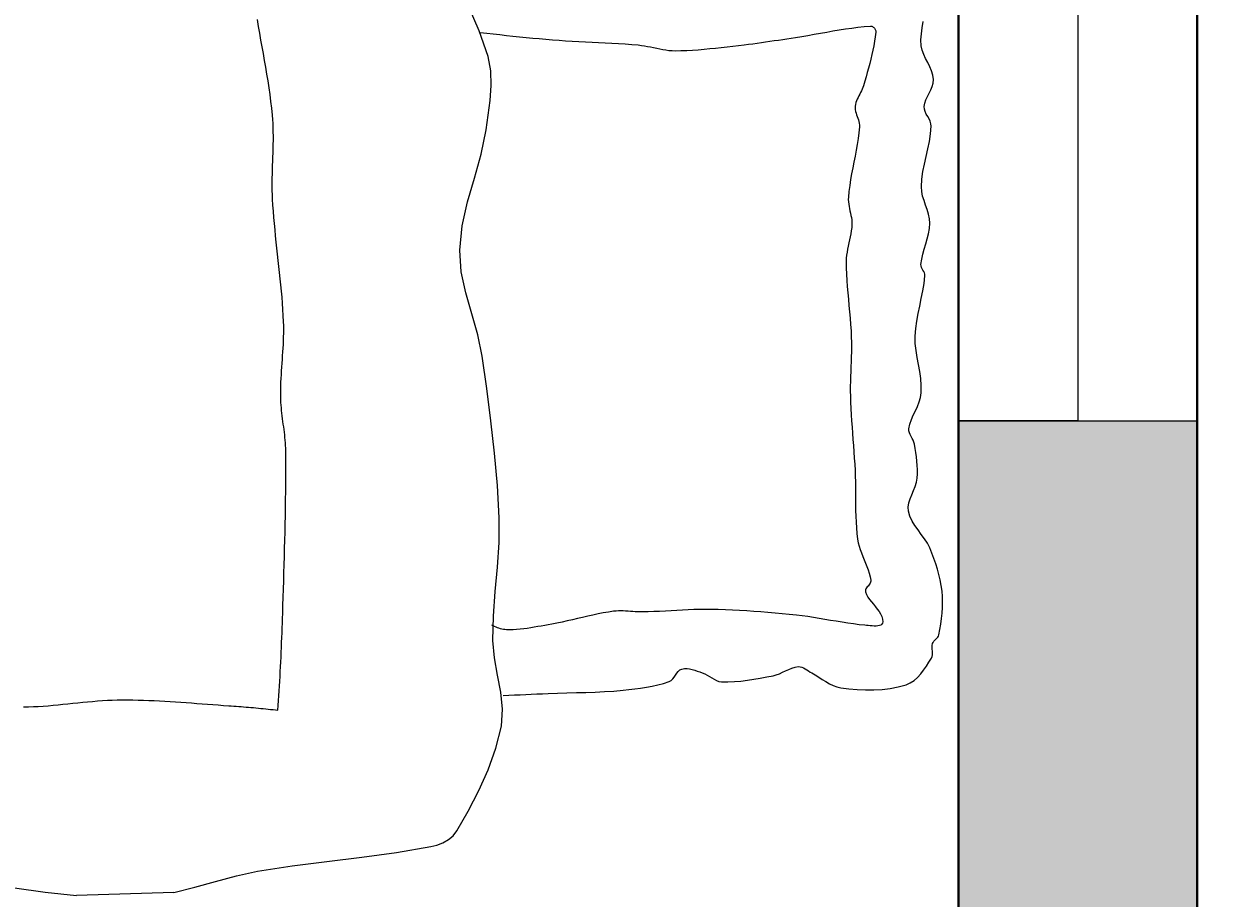
# Model space of a CAD drawing. Units: inches. Extents: x 1441 to 2460, y 1648 to 2683.
# Tile 16 of 35: x 1845 to 1890, y 2058 to 2091. Entities that reach past the tile are written whole.
import ezdxf

# ---------------------------------------------------------------- set-up
doc = ezdxf.new("R2010")
doc.units = ezdxf.units.IN
for name, color, linetype, lineweight in [('A-ANNO-DIMS', 2, 'Continuous', 18), ('A-FURN', 8, 'Continuous', 15), ('A-GLAZ', 4, 'Continuous', 18), ('A-WALL', 7, 'Continuous', 40)]:
    doc.layers.add(name, color=color, linetype=linetype, lineweight=lineweight)
doc.layers.add('A-WALL-PATT', color=251, linetype='Continuous', lineweight=13, true_color=0x636466)
doc.styles.get("Standard").update_dxf_attribs({"font": 'arial.ttf'})
doc.dimstyles.get("Standard").update_dxf_attribs({"dimtxt": 0.18, "dimasz": 0.18, "dimexe": 0.18, "dimexo": 0.0625, "dimgap": 0.09, "dimtad": 0, "dimtih": 1, "dimtoh": 1, "dimdec": 4, "dimzin": 0, "dimdsep": 46, "dimtxsty": 'Standard', "dimcen": 0.09, "dimadec": 0, "dimazin": 0, "dimtfac": 1, "dimtdec": 4, "dimtofl": 0, "dimtmove": 0, "dimatfit": 3, "dimfxl": 1, "dimtolj": 1, "dimtzin": 0, "dimarcsym": 0})

# ---------------------------------------------------------------- blocks, each defined once
blk = doc.blocks.new('BED-DOUBLE-PLAN')
for p, q in [((33.569, 91.32), (33.41, 91.271)), ((33.735, 91.343), (33.569, 91.32)), ((33.867, 91.333), (33.735, 91.343)), ((33.995, 91.298), (33.867, 91.333)), ((34.121, 91.245), (33.995, 91.298)), ((51.797, 91.361), (51.599, 91.285)), ((51.997, 91.432), (51.797, 91.361)), ((52.2, 91.497), (51.997, 91.432)), ((52.404, 91.554), (52.2, 91.497)), ((52.61, 91.603), (52.404, 91.554)), ((52.818, 91.642), (52.61, 91.603)), ((53.027, 91.67), (52.818, 91.642)), ((53.234, 91.686), (53.027, 91.67)), ((53.441, 91.69), (53.234, 91.686)), ((53.649, 91.684), (53.441, 91.69)), ((53.857, 91.67), (53.649, 91.684)), ((54.065, 91.648), (53.857, 91.67)), ((54.272, 91.619), (54.065, 91.648)), ((54.478, 91.587), (54.272, 91.619)), ((54.683, 91.551), (54.478, 91.587)), ((54.729, 91.535), (54.683, 91.551)), ((54.771, 91.509), (54.729, 91.535)), ((54.81, 91.475), (54.771, 91.509)), ((54.847, 91.437), (54.81, 91.475)), ((54.884, 91.398), (54.847, 91.437)), ((54.922, 91.361), (54.884, 91.398)), ((54.963, 91.331), (54.922, 91.361)), ((55.008, 91.31), (54.963, 91.331)), ((55.076, 91.296), (55.008, 91.31)), ((55.147, 91.294), (55.076, 91.296)), ((55.219, 91.299), (55.147, 91.294)), ((55.292, 91.306), (55.219, 91.299)), ((55.364, 91.311), (55.292, 91.306)), ((55.433, 91.31), (55.364, 91.311)), ((55.499, 91.298), (55.433, 91.31)), ((55.56, 91.27), (55.499, 91.298)), ((31.78, 90.922), (31.549, 90.959)), ((32.011, 90.889), (31.78, 90.922)), ((32.24, 90.873), (32.011, 90.889)), ((32.466, 90.885), (32.24, 90.873)), ((32.63, 90.922), (32.466, 90.885)), ((32.789, 90.98), (32.63, 90.922)), ((32.945, 91.051), (32.789, 90.98)), ((33.099, 91.129), (32.945, 91.051)), ((33.253, 91.205), (33.099, 91.129)), ((33.41, 91.271), (33.253, 91.205)), ((34.245, 91.181), (34.121, 91.245)), ((34.37, 91.117), (34.245, 91.181)), ((34.495, 91.058), (34.37, 91.117)), ((34.624, 91.015), (34.495, 91.058)), ((34.756, 90.994), (34.624, 91.015)), ((34.852, 91.003), (34.756, 90.994)), ((34.945, 91.032), (34.852, 91.003)), ((35.036, 91.076), (34.945, 91.032)), ((35.126, 91.127), (35.036, 91.076)), ((35.216, 91.178), (35.126, 91.127)), ((35.307, 91.222), (35.216, 91.178)), ((35.4, 91.252), (35.307, 91.222)), ((35.496, 91.261), (35.4, 91.252)), ((35.784, 91.238), (35.496, 91.261)), ((36.07, 91.194), (35.784, 91.238)), ((36.354, 91.135), (36.07, 91.194)), ((36.638, 91.07), (36.354, 91.135)), ((36.922, 91.006), (36.638, 91.07)), ((37.206, 90.949), (36.922, 91.006)), ((37.492, 90.908), (37.206, 90.949)), ((37.78, 90.89), (37.492, 90.908)), ((37.955, 90.902), (37.78, 90.89)), ((38.128, 90.938), (37.955, 90.902)), ((38.299, 90.989), (38.128, 90.938)), ((38.469, 91.048), (38.299, 90.989)), ((38.639, 91.107), (38.469, 91.048)), ((38.81, 91.159), (38.639, 91.107)), ((38.983, 91.195), (38.81, 91.159)), ((39.158, 91.208), (38.983, 91.195)), ((39.356, 91.195), (39.158, 91.208)), ((39.551, 91.161), (39.356, 91.195)), ((39.744, 91.114), (39.551, 91.161)), ((39.936, 91.058), (39.744, 91.114)), ((40.129, 91), (39.936, 91.058)), ((40.322, 90.946), (40.129, 91)), ((40.516, 90.901), (40.322, 90.946)), ((40.713, 90.873), (40.516, 90.901)), ((40.767, 90.876), (40.713, 90.873)), ((40.821, 90.893), (40.767, 90.876)), ((40.873, 90.918), (40.821, 90.893)), ((40.924, 90.949), (40.873, 90.918)), ((40.975, 90.979), (40.924, 90.949)), ((41.027, 91.005), (40.975, 90.979)), ((41.081, 91.022), (41.027, 91.005)), ((41.135, 91.025), (41.081, 91.022)), ((41.423, 90.993), (41.135, 91.025)), ((41.708, 90.945), (41.423, 90.993)), ((41.993, 90.887), (41.708, 90.945)), ((42.277, 90.826), (41.993, 90.887)), ((45.014, 90.865), (44.748, 90.826)), ((45.28, 90.887), (45.014, 90.865)), ((45.546, 90.884), (45.28, 90.887)), ((45.723, 90.857), (45.546, 90.884)), ((45.894, 90.807), (45.723, 90.857)), ((50.888, 90.886), (50.723, 90.763)), ((51.053, 91.006), (50.888, 90.886)), ((51.224, 91.115), (51.053, 91.006)), ((51.403, 91.204), (51.224, 91.115)), ((51.599, 91.285), (51.403, 91.204)), ((55.709, 91.176), (55.56, 91.27)), ((55.86, 91.078), (55.709, 91.176)), ((56.01, 90.975), (55.86, 91.078)), ((56.153, 90.865), (56.01, 90.975)), ((56.284, 90.746), (56.153, 90.865)), ((42.561, 90.766), (42.277, 90.826)), ((42.845, 90.714), (42.561, 90.766)), ((43.131, 90.675), (42.845, 90.714)), ((43.419, 90.654), (43.131, 90.675)), ((43.686, 90.66), (43.419, 90.654)), ((43.952, 90.687), (43.686, 90.66)), ((44.218, 90.73), (43.952, 90.687)), ((44.483, 90.779), (44.218, 90.73)), ((44.748, 90.826), (44.483, 90.779)), ((46.062, 90.739), (45.894, 90.807)), ((46.228, 90.663), (46.062, 90.739)), ((46.394, 90.585), (46.228, 90.663)), ((46.562, 90.514), (46.394, 90.585)), ((46.733, 90.456), (46.562, 90.514)), ((46.908, 90.42), (46.733, 90.456)), ((46.984, 90.419), (46.908, 90.42)), ((47.057, 90.436), (46.984, 90.419)), ((47.128, 90.465), (47.057, 90.436)), ((47.199, 90.502), (47.128, 90.465)), ((47.27, 90.541), (47.199, 90.502)), ((47.342, 90.578), (47.27, 90.541)), ((47.415, 90.609), (47.342, 90.578)), ((47.49, 90.629), (47.415, 90.609)), ((47.648, 90.655), (47.49, 90.629)), ((47.807, 90.68), (47.648, 90.655)), ((47.967, 90.702), (47.807, 90.68)), ((48.127, 90.721), (47.967, 90.702)), ((48.287, 90.734), (48.127, 90.721)), ((48.447, 90.741), (48.287, 90.734)), ((48.607, 90.741), (48.447, 90.741)), ((48.767, 90.731), (48.607, 90.741)), ((48.926, 90.703), (48.767, 90.731)), ((49.084, 90.654), (48.926, 90.703)), ((49.24, 90.592), (49.084, 90.654)), ((49.395, 90.526), (49.24, 90.592)), ((49.549, 90.466), (49.395, 90.526)), ((49.704, 90.42), (49.549, 90.466)), ((49.861, 90.397), (49.704, 90.42)), ((50.019, 90.406), (49.861, 90.397)), ((50.209, 90.459), (50.019, 90.406)), ((50.387, 90.542), (50.209, 90.459)), ((50.558, 90.646), (50.387, 90.542)), ((50.723, 90.763), (50.558, 90.646)), ((56.399, 90.616), (56.284, 90.746)), ((56.493, 90.473), (56.399, 90.616)), ((56.561, 90.317), (56.493, 90.473)), ((56.643, 90.02), (56.561, 90.317)), ((56.701, 89.716), (56.643, 90.02)), ((56.736, 89.408), (56.701, 89.716)), ((31.729, 89.025), (31.74, 89.05)), ((31.74, 89.05), (31.755, 89.074)), ((31.755, 89.074), (31.774, 89.097)), ((31.774, 89.097), (31.795, 89.117)), ((31.795, 89.117), (31.818, 89.136)), ((31.818, 89.136), (31.843, 89.151)), ((31.843, 89.151), (31.869, 89.163)), ((31.869, 89.163), (31.896, 89.172)), ((31.896, 89.172), (31.922, 89.176)), ((31.922, 89.176), (31.948, 89.176)), ((31.948, 89.176), (32.119, 89.153)), ((32.119, 89.153), (32.29, 89.126)), ((32.29, 89.126), (32.459, 89.095)), ((32.459, 89.095), (32.629, 89.06)), ((32.629, 89.06), (32.797, 89.023)), ((53.438, 89.006), (53.527, 89.081)), ((53.527, 89.081), (53.616, 89.156)), ((53.616, 89.156), (53.705, 89.228)), ((53.705, 89.228), (53.796, 89.294)), ((53.796, 89.294), (53.889, 89.351)), ((53.889, 89.351), (53.985, 89.396)), ((53.985, 89.396), (54.086, 89.424)), ((54.086, 89.424), (54.192, 89.433)), ((54.192, 89.433), (54.243, 89.423)), ((54.243, 89.423), (54.282, 89.397)), ((54.282, 89.397), (54.31, 89.358)), ((54.31, 89.358), (54.329, 89.307)), ((54.329, 89.307), (54.341, 89.247)), ((54.341, 89.247), (54.346, 89.18)), ((54.346, 89.109), (54.342, 89.035)), ((54.346, 89.18), (54.346, 89.109)), ((56.752, 89.096), (56.736, 89.408)), ((56.751, 88.783), (56.752, 89.096)), ((31.722, 88.975), (31.723, 89)), ((31.741, 88.737), (31.722, 88.975)), ((31.723, 89), (31.729, 89.025)), ((31.765, 88.499), (31.741, 88.737)), ((32.797, 89.023), (32.966, 88.982)), ((32.966, 88.982), (33.133, 88.94)), ((33.133, 88.94), (33.301, 88.895)), ((33.301, 88.895), (33.468, 88.85)), ((33.468, 88.85), (33.635, 88.803)), ((33.635, 88.803), (33.801, 88.756)), ((33.801, 88.756), (33.968, 88.709)), ((33.968, 88.709), (34.034, 88.688)), ((34.034, 88.688), (34.099, 88.662)), ((34.099, 88.662), (34.162, 88.632)), ((34.162, 88.632), (34.225, 88.599)), ((34.225, 88.599), (34.288, 88.566)), ((51.463, 88.586), (51.591, 88.632)), ((51.591, 88.632), (51.719, 88.683)), ((51.719, 88.683), (51.846, 88.735)), ((51.846, 88.735), (51.972, 88.787)), ((51.972, 88.787), (52.1, 88.838)), ((52.1, 88.838), (52.228, 88.885)), ((52.228, 88.885), (52.357, 88.926)), ((52.357, 88.926), (52.488, 88.961)), ((52.488, 88.961), (52.621, 88.986)), ((52.621, 88.986), (52.66, 88.986)), ((52.66, 88.986), (52.697, 88.976)), ((52.697, 88.976), (52.734, 88.958)), ((52.734, 88.958), (52.769, 88.934)), ((52.769, 88.934), (52.804, 88.906)), ((52.804, 88.906), (52.839, 88.877)), ((52.839, 88.877), (52.873, 88.848)), ((52.873, 88.848), (52.908, 88.822)), ((52.908, 88.822), (52.943, 88.8)), ((52.943, 88.8), (52.979, 88.785)), ((52.979, 88.785), (53.015, 88.778)), ((53.015, 88.778), (53.053, 88.783)), ((53.053, 88.783), (53.155, 88.821)), ((53.155, 88.821), (53.253, 88.873)), ((53.253, 88.873), (53.347, 88.936)), ((53.347, 88.936), (53.438, 89.006)), ((54.315, 88.761), (54.295, 88.544)), ((54.321, 88.821), (54.315, 88.761)), ((54.328, 88.889), (54.321, 88.821)), ((54.335, 88.961), (54.328, 88.889)), ((54.342, 89.035), (54.335, 88.961)), ((56.736, 88.47), (56.751, 88.783)), ((31.795, 88.263), (31.765, 88.499)), ((31.829, 88.027), (31.795, 88.263)), ((34.288, 88.566), (34.35, 88.532)), ((34.35, 88.532), (34.413, 88.5)), ((34.413, 88.5), (34.476, 88.469)), ((34.476, 88.469), (34.54, 88.442)), ((34.54, 88.442), (34.605, 88.419)), ((34.605, 88.419), (34.671, 88.401)), ((34.671, 88.401), (34.739, 88.39)), ((34.739, 88.39), (34.805, 88.388)), ((34.805, 88.388), (34.87, 88.394)), ((34.87, 88.394), (34.935, 88.407)), ((34.935, 88.407), (35, 88.425)), ((35, 88.425), (35.064, 88.446)), ((35.064, 88.446), (35.128, 88.468)), ((35.128, 88.468), (35.193, 88.491)), ((35.193, 88.491), (35.257, 88.513)), ((35.257, 88.513), (35.322, 88.531)), ((35.322, 88.531), (35.387, 88.545)), ((35.387, 88.545), (35.452, 88.552)), ((35.452, 88.552), (35.518, 88.552)), ((35.518, 88.552), (35.741, 88.531)), ((35.741, 88.531), (35.963, 88.503)), ((35.963, 88.503), (36.184, 88.469)), ((36.184, 88.469), (36.405, 88.43)), ((36.405, 88.43), (36.626, 88.388)), ((36.626, 88.388), (36.847, 88.345)), ((36.847, 88.345), (37.067, 88.302)), ((37.067, 88.302), (37.288, 88.26)), ((37.288, 88.26), (37.509, 88.221)), ((37.509, 88.221), (37.73, 88.187)), ((37.73, 88.187), (37.953, 88.158)), ((37.953, 88.158), (38.176, 88.137)), ((38.262, 88.134), (38.347, 88.138)), ((38.347, 88.138), (38.433, 88.148)), ((38.433, 88.148), (38.518, 88.162)), ((38.518, 88.162), (38.604, 88.178)), ((38.604, 88.178), (38.689, 88.197)), ((38.689, 88.197), (38.774, 88.216)), ((38.774, 88.216), (38.86, 88.233)), ((38.86, 88.233), (38.945, 88.249)), ((38.945, 88.249), (39.031, 88.261)), ((39.031, 88.261), (39.117, 88.268)), ((39.117, 88.268), (39.203, 88.268)), ((39.203, 88.268), (39.32, 88.261)), ((39.32, 88.261), (39.437, 88.247)), ((39.437, 88.247), (39.553, 88.228)), ((39.553, 88.228), (39.668, 88.206)), ((39.668, 88.206), (39.783, 88.181)), ((39.783, 88.181), (39.899, 88.155)), ((39.899, 88.155), (40.014, 88.13)), ((42.023, 88.137), (42.261, 88.16)), ((42.261, 88.16), (42.499, 88.183)), ((42.499, 88.183), (42.737, 88.204)), ((42.737, 88.204), (42.975, 88.222)), ((42.975, 88.222), (43.213, 88.237)), ((43.213, 88.237), (43.451, 88.247)), ((43.451, 88.247), (43.636, 88.251)), ((43.636, 88.251), (43.822, 88.251)), ((43.822, 88.251), (44.007, 88.249)), ((44.007, 88.249), (44.192, 88.244)), ((44.192, 88.244), (44.377, 88.238)), ((44.377, 88.238), (44.562, 88.231)), ((44.562, 88.231), (44.748, 88.224)), ((44.748, 88.224), (44.933, 88.217)), ((44.933, 88.217), (45.118, 88.212)), ((45.118, 88.212), (45.303, 88.209)), ((45.303, 88.209), (45.488, 88.209)), ((45.488, 88.209), (45.674, 88.212)), ((45.674, 88.212), (45.907, 88.22)), ((45.907, 88.22), (46.141, 88.231)), ((46.141, 88.231), (46.375, 88.244)), ((46.375, 88.244), (46.609, 88.259)), ((46.609, 88.259), (46.842, 88.275)), ((46.842, 88.275), (47.076, 88.292)), ((47.076, 88.292), (47.309, 88.309)), ((47.309, 88.309), (47.543, 88.327)), ((47.543, 88.327), (47.776, 88.344)), ((47.776, 88.344), (48.01, 88.36)), ((48.01, 88.36), (48.243, 88.374)), ((48.243, 88.374), (48.477, 88.387)), ((48.477, 88.387), (48.693, 88.396)), ((48.693, 88.396), (48.91, 88.401)), ((48.91, 88.401), (49.126, 88.404)), ((49.126, 88.404), (49.343, 88.405)), ((49.343, 88.405), (49.56, 88.406)), ((49.56, 88.406), (49.776, 88.407)), ((49.776, 88.407), (49.993, 88.41)), ((49.993, 88.41), (50.209, 88.415)), ((50.209, 88.415), (50.425, 88.425)), ((50.425, 88.425), (50.64, 88.439)), ((50.64, 88.439), (50.855, 88.459)), ((50.855, 88.459), (51.07, 88.486)), ((51.07, 88.486), (51.203, 88.511)), ((51.203, 88.511), (51.334, 88.544)), ((51.334, 88.544), (51.463, 88.586)), ((54.269, 88.328), (54.239, 88.112)), ((54.295, 88.544), (54.269, 88.328)), ((56.674, 87.849), (56.709, 88.158)), ((56.709, 88.158), (56.736, 88.47)), ((31.866, 87.791), (31.829, 88.027)), ((31.905, 87.555), (31.866, 87.791)), ((38.176, 88.137), (38.262, 88.134)), ((40.014, 88.13), (40.13, 88.106)), ((40.13, 88.106), (40.245, 88.085)), ((40.245, 88.085), (40.361, 88.069)), ((40.361, 88.069), (40.478, 88.058)), ((40.478, 88.058), (40.595, 88.053)), ((40.595, 88.053), (40.833, 88.055)), ((40.833, 88.055), (41.071, 88.064)), ((41.071, 88.064), (41.309, 88.077)), ((41.309, 88.077), (41.547, 88.095)), ((41.547, 88.095), (41.785, 88.115)), ((41.785, 88.115), (42.023, 88.137)), ((54.205, 87.897), (54.169, 87.682)), ((54.239, 88.112), (54.205, 87.897)), ((56.591, 87.558), (56.643, 87.7)), ((56.643, 87.7), (56.674, 87.849)), ((31.946, 87.319), (31.905, 87.555)), ((31.988, 87.084), (31.946, 87.319)), ((54.094, 87.252), (54.057, 87.037)), ((54.132, 87.467), (54.094, 87.252)), ((54.169, 87.682), (54.132, 87.467)), ((56.359, 87.153), (56.444, 87.286)), ((56.444, 87.286), (56.523, 87.42)), ((56.523, 87.42), (56.591, 87.558)), ((32.03, 86.849), (31.988, 87.084)), ((32.071, 86.613), (32.03, 86.849)), ((54.021, 86.822), (53.988, 86.607)), ((54.057, 87.037), (54.021, 86.822)), ((56.114, 86.752), (56.189, 86.888)), ((56.189, 86.888), (56.272, 87.021)), ((56.272, 87.021), (56.359, 87.153)), ((32.11, 86.377), (32.071, 86.613)), ((32.146, 86.141), (32.11, 86.377)), ((53.959, 86.391), (53.934, 86.174)), ((53.988, 86.607), (53.959, 86.391)), ((55.881, 86.316), (55.898, 86.382)), ((55.898, 86.382), (55.925, 86.445)), ((55.925, 86.445), (55.96, 86.507)), ((55.96, 86.507), (56, 86.568)), ((56, 86.568), (56.041, 86.629)), ((56.041, 86.629), (56.08, 86.69)), ((56.08, 86.69), (56.114, 86.752)), ((32.17, 85.981), (32.146, 86.141)), ((32.195, 85.82), (32.17, 85.981)), ((53.907, 85.907), (53.881, 85.64)), ((53.934, 86.174), (53.907, 85.907)), ((55.878, 86.248), (55.881, 86.316)), ((55.897, 86.124), (55.878, 86.248)), ((55.933, 86.004), (55.897, 86.124)), ((55.98, 85.887), (55.933, 86.004)), ((32.22, 85.659), (32.195, 85.82)), ((32.245, 85.499), (32.22, 85.659)), ((32.269, 85.338), (32.245, 85.499)), ((53.881, 85.64), (53.857, 85.373)), ((56.034, 85.771), (55.98, 85.887)), ((56.09, 85.655), (56.034, 85.771)), ((56.144, 85.538), (56.09, 85.655)), ((56.189, 85.419), (56.144, 85.538)), ((32.294, 85.177), (32.269, 85.338)), ((32.318, 85.017), (32.294, 85.177)), ((32.342, 84.856), (32.318, 85.017)), ((53.834, 85.105), (53.813, 84.838)), ((53.857, 85.373), (53.834, 85.105)), ((56.221, 85.297), (56.189, 85.419)), ((56.268, 85.056), (56.221, 85.297)), ((56.313, 84.813), (56.268, 85.056)), ((32.364, 84.695), (32.342, 84.856)), ((32.385, 84.534), (32.364, 84.695)), ((53.793, 84.57), (53.775, 84.302)), ((53.813, 84.838), (53.793, 84.57)), ((56.355, 84.57), (56.313, 84.813)), ((56.391, 84.327), (56.355, 84.57)), ((32.406, 84.372), (32.385, 84.534)), ((32.424, 84.211), (32.406, 84.372)), ((32.449, 83.994), (32.424, 84.211)), ((53.775, 84.302), (53.76, 84.034)), ((56.42, 84.082), (56.391, 84.327)), ((32.474, 83.778), (32.449, 83.994)), ((32.499, 83.561), (32.474, 83.778)), ((53.746, 83.766), (53.735, 83.498)), ((53.76, 84.034), (53.746, 83.766)), ((56.44, 83.838), (56.42, 84.082)), ((56.45, 83.593), (56.44, 83.838)), ((32.524, 83.344), (32.499, 83.561)), ((32.549, 83.127), (32.524, 83.344)), ((53.725, 83.23), (53.719, 82.961)), ((53.735, 83.498), (53.725, 83.23)), ((56.4, 83.159), (56.432, 83.251)), ((56.432, 83.251), (56.446, 83.348)), ((56.446, 83.348), (56.45, 83.593)), ((32.571, 82.909), (32.549, 83.127)), ((32.592, 82.692), (32.571, 82.909)), ((53.719, 82.961), (53.717, 82.745)), ((53.717, 82.745), (53.719, 82.529)), ((56.146, 82.721), (56.194, 82.81)), ((56.194, 82.81), (56.248, 82.897)), ((56.248, 82.897), (56.304, 82.983)), ((56.304, 82.983), (56.356, 83.07)), ((56.356, 83.07), (56.4, 83.159)), ((32.61, 82.475), (32.592, 82.692)), ((32.625, 82.257), (32.61, 82.475)), ((53.719, 82.529), (53.725, 82.313)), ((53.725, 82.313), (53.733, 82.097)), ((55.983, 82.246), (56.011, 82.343)), ((56.011, 82.343), (56.043, 82.439)), ((56.043, 82.439), (56.077, 82.535)), ((56.077, 82.535), (56.108, 82.628)), ((56.108, 82.628), (56.146, 82.721)), ((32.637, 82.04), (32.625, 82.257)), ((32.645, 81.822), (32.637, 82.04)), ((53.733, 82.097), (53.743, 81.881)), ((53.743, 81.881), (53.755, 81.665)), ((55.95, 82.052), (55.961, 82.149)), ((55.951, 81.956), (55.95, 82.052)), ((55.967, 81.861), (55.951, 81.956)), ((55.961, 82.149), (55.983, 82.246)), ((56.001, 81.786), (55.967, 81.861)), ((32.635, 81.37), (32.644, 81.487)), ((32.644, 81.487), (32.648, 81.604)), ((32.648, 81.604), (32.645, 81.822)), ((53.755, 81.665), (53.768, 81.449)), ((53.768, 81.449), (53.78, 81.233)), ((56.055, 81.723), (56.001, 81.786)), ((56.122, 81.667), (56.055, 81.723)), ((56.197, 81.616), (56.122, 81.667)), ((56.273, 81.564), (56.197, 81.616)), ((56.343, 81.51), (56.273, 81.564)), ((56.401, 81.448), (56.343, 81.51)), ((56.441, 81.375), (56.401, 81.448)), ((32.556, 80.908), (32.58, 81.023)), ((32.58, 81.023), (32.602, 81.139)), ((32.602, 81.139), (32.62, 81.254)), ((32.62, 81.254), (32.635, 81.37)), ((53.78, 81.233), (53.792, 81.017)), ((53.792, 81.017), (53.803, 80.801)), ((56.51, 81.165), (56.441, 81.375)), ((56.568, 80.953), (56.51, 81.165)), ((56.617, 80.737), (56.568, 80.953)), ((32.463, 80.445), (32.484, 80.561)), ((32.484, 80.561), (32.507, 80.677)), ((32.507, 80.677), (32.532, 80.792)), ((32.532, 80.792), (32.556, 80.908)), ((53.803, 80.801), (53.812, 80.585)), ((53.812, 80.585), (53.817, 80.369)), ((56.657, 80.52), (56.617, 80.737)), ((56.691, 80.301), (56.657, 80.52)), ((32.412, 79.964), (32.433, 80.213)), ((32.433, 80.213), (32.446, 80.329)), ((32.446, 80.329), (32.463, 80.445)), ((53.81, 80.097), (53.803, 80.007)), ((53.815, 80.188), (53.81, 80.097)), ((53.817, 80.278), (53.815, 80.188)), ((53.817, 80.369), (53.817, 80.278)), ((56.72, 80.081), (56.691, 80.301)), ((56.745, 79.861), (56.72, 80.081)), ((32.379, 79.466), (32.394, 79.715)), ((32.394, 79.715), (32.412, 79.964)), ((53.778, 79.644), (53.776, 79.554)), ((53.782, 79.735), (53.778, 79.644)), ((53.789, 79.825), (53.782, 79.735)), ((53.796, 79.916), (53.789, 79.825)), ((53.803, 80.007), (53.796, 79.916)), ((56.767, 79.641), (56.745, 79.861)), ((56.798, 79.289), (56.767, 79.641)), ((32.353, 78.967), (32.365, 79.217)), ((32.365, 79.217), (32.379, 79.466)), ((53.776, 79.554), (53.776, 79.464)), ((53.776, 79.464), (53.781, 79.374)), ((53.781, 79.374), (53.791, 79.284)), ((53.791, 79.284), (53.819, 79.088)), ((56.82, 78.937), (56.798, 79.289)), ((32.33, 78.469), (32.341, 78.718)), ((32.341, 78.718), (32.353, 78.967)), ((53.819, 79.088), (53.853, 78.892)), ((53.853, 78.892), (53.891, 78.697)), ((53.891, 78.697), (53.932, 78.503)), ((56.836, 78.584), (56.82, 78.937)), ((32.318, 78.219), (32.33, 78.469)), ((53.932, 78.503), (53.975, 78.309)), ((53.975, 78.309), (54.019, 78.115)), ((56.848, 78.231), (56.836, 78.584)), ((32.291, 77.721), (32.305, 77.97)), ((32.305, 77.97), (32.318, 78.219)), ((54.019, 78.115), (54.065, 77.922)), ((54.065, 77.922), (54.11, 77.728)), ((56.857, 77.878), (56.848, 78.231)), ((56.866, 77.524), (56.857, 77.878)), ((32.257, 77.223), (32.275, 77.472)), ((32.275, 77.472), (32.291, 77.721)), ((54.11, 77.728), (54.154, 77.534)), ((54.154, 77.534), (54.197, 77.34)), ((56.876, 77.171), (56.866, 77.524)), ((32.215, 76.726), (32.237, 76.974)), ((32.237, 76.974), (32.257, 77.223)), ((54.197, 77.34), (54.237, 77.145)), ((54.237, 77.145), (54.274, 76.95)), ((54.274, 76.95), (54.298, 76.818)), ((56.89, 76.818), (56.876, 77.171)), ((32.17, 76.23), (32.193, 76.478)), ((32.193, 76.478), (32.215, 76.726)), ((54.298, 76.818), (54.322, 76.686)), ((54.322, 76.686), (54.346, 76.554)), ((54.346, 76.554), (54.37, 76.421)), ((56.899, 76.605), (56.89, 76.818)), ((56.908, 76.392), (56.899, 76.605)), ((32.147, 75.981), (32.17, 76.23)), ((54.37, 76.421), (54.393, 76.289)), ((54.393, 76.289), (54.414, 76.156)), ((54.414, 76.156), (54.434, 76.023)), ((54.434, 76.023), (54.451, 75.89)), ((56.918, 76.179), (56.908, 76.392)), ((56.928, 75.966), (56.918, 76.179)), ((32.097, 75.486), (32.122, 75.733)), ((32.122, 75.733), (32.147, 75.981)), ((54.451, 75.89), (54.466, 75.757)), ((54.466, 75.757), (54.478, 75.624)), ((54.478, 75.624), (54.486, 75.49)), ((56.937, 75.753), (56.928, 75.966)), ((56.947, 75.54), (56.937, 75.753)), ((32.043, 74.99), (32.07, 75.238)), ((32.07, 75.238), (32.097, 75.486)), ((54.472, 75.126), (54.461, 75.069)), ((54.481, 75.184), (54.472, 75.126)), ((54.487, 75.241), (54.481, 75.184)), ((54.486, 75.49), (54.49, 75.356)), ((54.49, 75.299), (54.487, 75.241)), ((54.49, 75.356), (54.49, 75.299)), ((57.484, 75.097), (56.84, 75.028)), ((56.957, 75.327), (56.947, 75.54)), ((56.967, 75.114), (56.957, 75.327)), ((58.123, 75.053), (57.484, 75.097)), ((31.986, 74.495), (32.015, 74.742)), ((32.015, 74.742), (32.043, 74.99)), ((33.405, 74.651), (32.864, 74.545)), ((33.96, 74.67), (33.405, 74.651)), ((34.522, 74.63), (33.96, 74.67)), ((46.604, 74.657), (45.387, 74.497)), ((47.824, 74.794), (46.604, 74.657)), ((49.046, 74.901), (47.824, 74.794)), ((50.27, 74.969), (49.046, 74.901)), ((51.196, 74.964), (50.27, 74.969)), ((52.121, 74.904), (51.196, 74.964)), ((53.045, 74.821), (52.121, 74.904)), ((53.971, 74.75), (53.045, 74.821)), ((54.897, 74.726), (53.971, 74.75)), ((54.34, 74.744), (54.311, 74.694)), ((54.366, 74.795), (54.34, 74.744)), ((54.39, 74.848), (54.366, 74.795)), ((54.411, 74.902), (54.39, 74.848)), ((54.43, 74.957), (54.411, 74.902)), ((54.447, 75.012), (54.43, 74.957)), ((54.461, 75.069), (54.447, 75.012)), ((55.545, 74.784), (54.897, 74.726)), ((56.194, 74.904), (55.545, 74.784)), ((56.84, 75.028), (56.194, 74.904)), ((58.956, 74.846), (58.123, 75.053)), ((59.766, 74.555), (58.956, 74.846)), ((31.901, 74.215), (30.964, 73.813)), ((32.864, 74.545), (31.901, 74.215)), ((31.956, 74.247), (31.986, 74.495)), ((35.083, 74.555), (34.522, 74.63)), ((35.638, 74.47), (35.083, 74.555)), ((36.55, 74.284), (35.638, 74.47)), ((37.452, 74.033), (36.55, 74.284)), ((44.172, 74.323), (43.37, 74.156)), ((45.387, 74.497), (44.172, 74.323)), ((60.555, 74.2), (59.766, 74.555)), ((61.324, 73.8), (60.555, 74.2)), ((38.351, 73.775), (37.452, 74.033)), ((39.257, 73.571), (38.351, 73.775)), ((42.576, 73.933), (41.783, 73.709)), ((43.37, 74.156), (42.576, 73.933)), ((62.074, 73.372), (61.324, 73.8)), ((40.176, 73.479), (39.257, 73.571)), ((40.985, 73.539), (40.176, 73.479)), ((41.783, 73.709), (40.985, 73.539)), ((62.255, 73.232), (62.074, 73.372)), ((62.403, 73.052), (62.255, 73.232)), ((62.52, 72.843), (62.403, 73.052)), ((62.608, 72.619), (62.52, 72.843)), ((62.667, 72.392), (62.608, 72.619)), ((62.893, 71.092), (62.667, 72.392)), ((63.068, 69.783), (62.893, 71.092)), ((63.223, 68.471), (63.068, 69.783)), ((63.387, 67.161), (63.223, 68.471)), ((63.59, 65.856), (63.387, 67.161)), ((39.863, 66.56), (39.632, 66.535)), ((40.094, 66.585), (39.863, 66.56)), ((40.325, 66.61), (40.094, 66.585)), ((40.556, 66.636), (40.325, 66.61)), ((40.787, 66.661), (40.556, 66.636)), ((41.018, 66.686), (40.787, 66.661)), ((41.25, 66.711), (41.018, 66.686)), ((41.481, 66.734), (41.25, 66.711)), ((41.712, 66.756), (41.481, 66.734)), ((41.944, 66.776), (41.712, 66.756)), ((42.175, 66.795), (41.944, 66.776)), ((42.407, 66.811), (42.175, 66.795)), ((42.639, 66.825), (42.407, 66.811)), ((42.871, 66.836), (42.639, 66.825)), ((43.013, 66.84), (42.871, 66.836)), ((43.155, 66.842), (43.013, 66.84)), ((43.298, 66.841), (43.155, 66.842)), ((43.44, 66.838), (43.298, 66.841)), ((43.582, 66.833), (43.44, 66.838)), ((43.724, 66.826), (43.582, 66.833)), ((43.867, 66.819), (43.724, 66.826)), ((44.009, 66.81), (43.867, 66.819)), ((44.151, 66.8), (44.009, 66.81)), ((44.294, 66.79), (44.151, 66.8)), ((44.436, 66.78), (44.294, 66.79)), ((44.578, 66.77), (44.436, 66.78)), ((44.72, 66.76), (44.578, 66.77)), ((44.863, 66.751), (44.72, 66.76)), ((45.005, 66.743), (44.863, 66.751)), ((45.147, 66.736), (45.005, 66.743)), ((45.29, 66.731), (45.147, 66.736)), ((45.432, 66.727), (45.29, 66.731)), ((45.574, 66.726), (45.432, 66.727)), ((45.717, 66.727), (45.574, 66.726)), ((45.818, 66.73), (45.717, 66.727)), ((45.92, 66.735), (45.818, 66.73)), ((46.021, 66.742), (45.92, 66.735)), ((46.122, 66.751), (46.021, 66.742)), ((46.223, 66.761), (46.122, 66.751)), ((46.324, 66.773), (46.223, 66.761)), ((46.425, 66.785), (46.324, 66.773)), ((46.526, 66.798), (46.425, 66.785)), ((46.627, 66.811), (46.526, 66.798)), ((46.727, 66.825), (46.627, 66.811)), ((46.828, 66.839), (46.727, 66.825)), ((46.929, 66.852), (46.828, 66.839)), ((47.03, 66.865), (46.929, 66.852)), ((47.131, 66.877), (47.03, 66.865)), ((47.232, 66.888), (47.131, 66.877)), ((47.333, 66.898), (47.232, 66.888)), ((47.434, 66.906), (47.333, 66.898)), ((47.535, 66.912), (47.434, 66.906)), ((47.637, 66.917), (47.535, 66.912)), ((47.738, 66.919), (47.637, 66.917)), ((48.045, 66.921), (47.738, 66.919)), ((48.352, 66.922), (48.045, 66.921)), ((48.658, 66.921), (48.352, 66.922)), ((48.965, 66.92), (48.658, 66.921)), ((49.272, 66.917), (48.965, 66.92)), ((49.579, 66.913), (49.272, 66.917)), ((49.885, 66.909), (49.579, 66.913)), ((50.192, 66.903), (49.885, 66.909)), ((50.499, 66.897), (50.192, 66.903)), ((50.806, 66.89), (50.499, 66.897)), ((51.112, 66.883), (50.806, 66.89)), ((51.419, 66.875), (51.112, 66.883)), ((51.726, 66.866), (51.419, 66.875)), ((52.032, 66.857), (51.726, 66.866)), ((52.339, 66.848), (52.032, 66.857)), ((52.646, 66.839), (52.339, 66.848)), ((52.952, 66.83), (52.646, 66.839)), ((53.259, 66.82), (52.952, 66.83)), ((53.566, 66.811), (53.259, 66.82)), ((53.872, 66.801), (53.566, 66.811)), ((54.055, 66.796), (53.872, 66.801)), ((54.237, 66.79), (54.055, 66.796)), ((54.42, 66.783), (54.237, 66.79)), ((54.602, 66.777), (54.42, 66.783)), ((54.785, 66.77), (54.602, 66.777)), ((54.967, 66.762), (54.785, 66.77)), ((55.15, 66.755), (54.967, 66.762)), ((55.332, 66.747), (55.15, 66.755)), ((55.515, 66.738), (55.332, 66.747)), ((55.697, 66.729), (55.515, 66.738)), ((55.879, 66.72), (55.697, 66.729)), ((56.062, 66.711), (55.879, 66.72)), ((56.244, 66.701), (56.062, 66.711)), ((56.426, 66.691), (56.244, 66.701)), ((56.609, 66.681), (56.426, 66.691)), ((56.791, 66.67), (56.609, 66.681)), ((56.973, 66.659), (56.791, 66.67)), ((57.155, 66.648), (56.973, 66.659)), ((57.338, 66.636), (57.155, 66.648)), ((57.52, 66.624), (57.338, 66.636)), ((57.509, 66.531), (57.52, 66.624)), ((33.016, 66.119), (32.759, 66.074)), ((33.273, 66.163), (33.016, 66.119)), ((33.53, 66.207), (33.273, 66.163)), ((33.787, 66.248), (33.53, 66.207)), ((34.045, 66.287), (33.787, 66.248)), ((34.303, 66.324), (34.045, 66.287)), ((34.561, 66.358), (34.303, 66.324)), ((34.82, 66.388), (34.561, 66.358)), ((35.079, 66.415), (34.82, 66.388)), ((35.237, 66.428), (35.079, 66.415)), ((35.394, 66.438), (35.237, 66.428)), ((35.552, 66.444), (35.394, 66.438)), ((35.71, 66.448), (35.552, 66.444)), ((35.868, 66.45), (35.71, 66.448)), ((36.026, 66.449), (35.868, 66.45)), ((36.184, 66.447), (36.026, 66.449)), ((36.343, 66.444), (36.184, 66.447)), ((36.501, 66.439), (36.343, 66.444)), ((36.66, 66.434), (36.501, 66.439)), ((36.818, 66.428), (36.66, 66.434)), ((36.976, 66.423), (36.818, 66.428)), ((37.135, 66.418), (36.976, 66.423)), ((37.293, 66.413), (37.135, 66.418)), ((37.451, 66.41), (37.293, 66.413)), ((37.61, 66.408), (37.451, 66.41)), ((37.768, 66.408), (37.61, 66.408)), ((37.926, 66.41), (37.768, 66.408)), ((38.084, 66.414), (37.926, 66.41)), ((38.242, 66.421), (38.084, 66.414)), ((38.474, 66.435), (38.242, 66.421)), ((38.706, 66.451), (38.474, 66.435)), ((38.938, 66.47), (38.706, 66.451)), ((39.169, 66.49), (38.938, 66.47)), ((39.4, 66.512), (39.169, 66.49)), ((39.632, 66.535), (39.4, 66.512)), ((57.46, 66.069), (57.469, 66.161)), ((57.469, 66.161), (57.479, 66.254)), ((57.479, 66.254), (57.489, 66.346)), ((57.489, 66.346), (57.499, 66.439)), ((57.499, 66.439), (57.509, 66.531)), ((31.732, 65.891), (31.475, 65.847)), ((31.989, 65.936), (31.732, 65.891)), ((32.246, 65.982), (31.989, 65.936)), ((32.502, 66.028), (32.246, 65.982)), ((32.759, 66.074), (32.502, 66.028)), ((57.416, 65.606), (57.425, 65.699)), ((57.425, 65.699), (57.433, 65.791)), ((57.433, 65.791), (57.442, 65.884)), ((57.442, 65.884), (57.451, 65.976)), ((57.451, 65.976), (57.46, 66.069)), ((63.763, 65.061), (63.59, 65.856)), ((57.378, 65.142), (57.385, 65.235)), ((57.385, 65.235), (57.393, 65.328)), ((57.393, 65.328), (57.4, 65.421)), ((57.4, 65.421), (57.408, 65.513)), ((57.408, 65.513), (57.416, 65.606)), ((57.338, 64.57), (57.352, 64.771)), ((57.352, 64.771), (57.358, 64.864)), ((57.358, 64.864), (57.364, 64.957)), ((57.364, 64.957), (57.371, 65.05)), ((57.371, 65.05), (57.378, 65.142)), ((63.975, 64.273), (63.763, 65.061)), ((57.309, 64.168), (57.324, 64.369)), ((57.324, 64.369), (57.338, 64.57)), ((57.278, 63.767), (57.294, 63.968)), ((57.294, 63.968), (57.309, 64.168)), ((64.196, 63.488), (63.975, 64.273)), ((57.248, 63.365), (57.263, 63.566)), ((57.263, 63.566), (57.278, 63.767)), ((64.395, 62.698), (64.196, 63.488)), ((57.204, 62.762), (57.218, 62.963)), ((57.218, 62.963), (57.233, 63.164)), ((57.233, 63.164), (57.248, 63.365)), ((57.179, 62.359), (57.191, 62.56)), ((57.191, 62.56), (57.204, 62.762)), ((64.395, 62.698), (64.503, 59.019)), ((57.157, 61.957), (57.168, 62.158)), ((57.168, 62.158), (57.179, 62.359)), ((57.141, 61.555), (57.149, 61.756)), ((57.149, 61.756), (57.157, 61.957)), ((57.132, 61.152), (57.136, 61.353)), ((57.136, 61.353), (57.141, 61.555)), ((57.13, 60.951), (57.132, 61.152)), ((57.13, 60.749), (57.13, 60.951)), ((57.133, 60.563), (57.13, 60.749)), ((57.139, 60.376), (57.133, 60.563)), ((57.147, 60.19), (57.139, 60.376)), ((57.159, 60.003), (57.147, 60.19)), ((57.172, 59.817), (57.159, 60.003)), ((57.188, 59.631), (57.172, 59.817)), ((57.205, 59.445), (57.188, 59.631)), ((57.222, 59.259), (57.205, 59.445)), ((57.241, 59.073), (57.222, 59.259)), ((57.26, 58.887), (57.241, 59.073)), ((64.382, 57.848), (64.503, 59.019)), ((57.279, 58.701), (57.26, 58.887)), ((57.298, 58.515), (57.279, 58.701)), ((57.317, 58.328), (57.298, 58.515)), ((57.334, 58.142), (57.317, 58.328)), ((57.35, 57.956), (57.334, 58.142)), ((57.364, 57.77), (57.35, 57.956)), ((57.377, 57.584), (57.364, 57.77)), ((57.387, 57.397), (57.377, 57.584)), ((64.222, 56.681), (64.382, 57.848)), ((57.394, 57.211), (57.387, 57.397)), ((57.398, 57.024), (57.394, 57.211))]:
    blk.add_line(p, q)
blk = doc.blocks.new('WIN-48-SASH')
for p, q in [((8.996, 48.001), (4.496, 48.001)), ((4.496, 48.001), (4.496, 0.001)), ((4.496, 0.001), (-0.004, 0.001))]:
    blk.add_line(p, q)
blk = doc.blocks.new('*D67')
at = {"layer": 'A-ANNO-DIMS', "color": 0, "lineweight": -2, "transparency": 16777216}
for p, q in [((1889.448, 2298.695), (1916.216, 2298.695)), ((1916.036, 2298.515), (1916.036, 2055.938)), ((1916.036, 1812.997), (1916.036, 2055.574)), ((1758.224, 1812.817), (1916.216, 1812.817))]:
    blk.add_line(p, q, dxfattribs=at)
at = {"layer": 'A-ANNO-DIMS', "color": 0, "transparency": 16777216}
for points in [[(1916.006, 2298.515), (1916.066, 2298.515), (1916.036, 2298.695)], [(1916.006, 1812.997), (1916.066, 1812.997), (1916.036, 1812.817)]]:
    blk.add_solid(points, dxfattribs=at)
at = {"layer": 'Defpoints', "color": 0, "transparency": 16777216}
for p in [(1889.386, 2298.695), (1916.036, 2298.695), (1758.161, 1812.817)]:
    blk.add_point(p, dxfattribs=at)
at = {"layer": 'A-ANNO-DIMS', "color": 0, "transparency": 16777216, "insert": (1916.036, 2055.756), "char_height": 0.18, "attachment_point": 5}
blk.add_mtext('\\A1;485.9', dxfattribs=at)

msp = doc.modelspace()

# ---------------------------------------------------------------- hatches: boundary and pattern name
at = {"layer": 'A-WALL-PATT'}
h = msp.add_hatch(color=256, dxfattribs=at)
h.dxf.hatch_style = 1
h.paths.add_polyline_path([(1627.5085, 2298.6952), (1568.8859, 2298.6952), (1568.8859, 2246.9605), (1577.8859, 2246.9605), (1577.8859, 2289.6952), (1627.5085, 2289.6952), (1627.5085, 2294.1952)])
h.paths.add_polyline_path([(1675.5777, 2298.6952), (1651.5085, 2298.6952), (1651.5085, 2289.6952), (1675.5777, 2289.6952), (1675.5777, 2294.1952)])
h.paths.add_polyline_path([(1667.3859, 2289.6952), (1662.8859, 2289.6952), (1662.8859, 2233.0622), (1667.3859, 2233.0622)])
h.paths.add_polyline_path([(1715.8721, 2294.3362), (1715.8721, 2295.2788), (1715.8721, 2298.6952), (1699.5777, 2298.6952), (1699.5777, 2289.6952), (1715.8721, 2289.6952)])
h.paths.add_polyline_path([(1707.8859, 2289.6952), (1703.3859, 2289.6952), (1703.3859, 2199.6952), (1707.8859, 2199.6952)])
h.paths.add_polyline_path([(1760.3859, 2204.637), (1755.8859, 2204.637), (1755.8859, 2199.6952), (1667.3859, 2199.6952), (1667.3859, 2204.637), (1662.8859, 2204.637), (1662.8859, 2195.1952), (1760.3859, 2195.1952)])
h.paths.add_polyline_path([(1760.3859, 2289.6952), (1755.8859, 2289.6952), (1755.8859, 2233.0622), (1760.3859, 2233.0622)])
h.paths.add_polyline_path([(1889.3859, 2298.6952), (1739.8721, 2298.6952), (1739.8721, 2289.6952), (1880.3859, 2289.6952), (1880.3859, 2250.8051), (1889.3859, 2250.8051)])
h.paths.add_polyline_path([(1889.3859, 2202.8051), (1880.3859, 2202.8051), (1880.3859, 2157.6952), (1747.948, 2157.6952), (1747.948, 2153.1952), (1755.8859, 2153.1952), (1755.8859, 2058.005), (1760.3859, 2058.005), (1760.3859, 2153.1952), (1880.3859, 2153.1952), (1880.3859, 2124.108), (1889.3859, 2124.108)])
h.paths.add_polyline_path([(1889.3859, 1984.8305), (1880.3859, 1984.8305), (1880.3859, 1834.1952), (1889.3859, 1834.1952)])
h.paths.add_polyline_path([(1889.3859, 2076.108), (1880.3859, 2076.108), (1880.3859, 2008.8305), (1889.3859, 2008.8305)])
h.paths.add_polyline_path([(1880.3859, 2027.1952), (1800.8859, 2027.1952), (1800.8859, 2000.9452), (1805.3859, 2000.9452), (1805.3859, 2022.6952), (1880.3859, 2022.6952)])
h.paths.add_polyline_path([(1800.8859, 2027.1952), (1760.3859, 2027.1952), (1760.3859, 2030.7912), (1755.8859, 2030.7912), (1755.8859, 2022.6952), (1800.8859, 2022.6952)])
h.paths.add_polyline_path([(1880.3859, 1974.6952), (1805.3859, 1974.6952), (1805.3859, 1978.7973), (1800.8859, 1978.7973), (1800.8859, 1974.6952), (1794.8823, 1974.6952), (1794.8823, 1970.1952), (1800.8859, 1970.1952), (1805.3859, 1970.1952), (1880.3859, 1970.1952)])
h.paths.add_polyline_path([(1760.3859, 1974.6952), (1755.8859, 1974.6952), (1755.8859, 1925.6952), (1751.8616, 1925.6952), (1751.8616, 1921.1952), (1760.3859, 1921.1952)])
h.paths.add_polyline_path([(1760.3859, 1921.1952), (1755.8859, 1921.1952), (1755.8859, 1843.1952), (1760.3859, 1843.1952)])
h.paths.add_polyline_path([(1799.1136, 1838.6952), (1799.1136, 1843.1952), (1760.3859, 1843.1952), (1751.8944, 1843.1952), (1751.8944, 1834.1952), (1758.1615, 1834.1952), (1799.1136, 1834.1952)])
h.paths.add_polyline_path([(1880.3859, 1843.1952), (1859.1136, 1843.1952), (1859.1136, 1834.1952), (1880.3859, 1834.1952)])
h.paths.add_polyline_path([(1577.8859, 1857.7914), (1568.8859, 1857.7914), (1568.8859, 1834.1952), (1695.0034, 1834.1952), (1695.0034, 1838.6952), (1695.0034, 1843.1952), (1577.8859, 1843.1952)])
h.paths.add_polyline_path([(1577.8859, 1959.2399), (1573.3859, 1959.2399), (1568.8859, 1959.2399), (1568.8859, 1905.7914), (1577.8859, 1905.7914), (1577.8859, 1921.1952), (1703.3859, 1921.1952), (1707.8859, 1921.1952), (1715.1501, 1921.1952), (1715.1501, 1925.6952), (1707.8859, 1925.6952), (1703.3859, 1925.6952), (1577.8859, 1925.6952)])
h.paths.add_polyline_path([(1577.8859, 2106.6907), (1568.8859, 2106.6907), (1568.8859, 2019.2399), (1577.8859, 2019.2399)])
h.paths.add_polyline_path([(1707.8859, 2051.6952), (1703.3859, 2051.6952), (1703.3859, 2048.6952), (1703.3859, 1925.6952), (1707.8859, 1925.6952)])
h.paths.add_polyline_path([(1703.3859, 2051.6952), (1676.3859, 2051.6952), (1676.3859, 2048.6952), (1703.3859, 2048.6952)])
h.paths.add_polyline_path([(1703.3859, 2102.6952), (1676.3859, 2102.6952), (1676.3859, 2099.6952), (1685.3859, 2099.6952), (1703.3859, 2099.6952)])
h.paths.add_polyline_path([(1707.8859, 2153.1952), (1710.5611, 2153.1952), (1710.5611, 2157.6952), (1707.8859, 2157.6952), (1707.8859, 2195.1952), (1703.3859, 2195.1952), (1703.3859, 2099.6952), (1707.8859, 2099.6952)])
h.paths.add_polyline_path([(1577.8859, 2198.9605), (1568.8859, 2198.9605), (1568.8859, 2166.6907), (1577.8859, 2166.6907)])

# ---------------------------------------------------------------- linework, layer by layer
at = {"layer": 'A-GLAZ'}
msp.add_line((1880.3859, 2076.108), (1889.3859, 2076.108), dxfattribs=at)
at = {"layer": 'A-WALL'}
for p, q in [((1889.3859, 2298.6952), (1889.3859, 1834.1952)), ((1880.3859, 2153.1952), (1880.3859, 1834.1952))]:
    msp.add_line(p, q, dxfattribs=at)

# ---------------------------------------------------------------- block references
at = {"layer": 'A-FURN', "rotation": 270}
msp.add_blockref('BED-DOUBLE-PLAN', (1788.0907, 2122.7206), dxfattribs=at)
at = {"layer": 'A-GLAZ'}
msp.add_blockref('WIN-48-SASH', (1880.39, 2076.1074), dxfattribs=at)

# ---------------------------------------------------------------- dimensions: what is measured, and where the dimension line sits
at = {"layer": 'A-ANNO-DIMS'}
dim = msp.add_linear_dim(base=(1916.0359, 2298.6952), p1=(1758.1615, 1812.8171), p2=(1889.3859, 2298.6952), angle=90, dimstyle='Standard', override={"dimdec": 1, "dimlfac": 1, "dimrnd": 0, "dimzin": 0, "dimdsep": 46, "dimlunit": 2}, dxfattribs=at)
dim.commit()
dim.dimension.update_dxf_attribs({"geometry": '*D67', "text_midpoint": (1916.0359, 2055.7561)})

doc.saveas('drawing.dxf')
